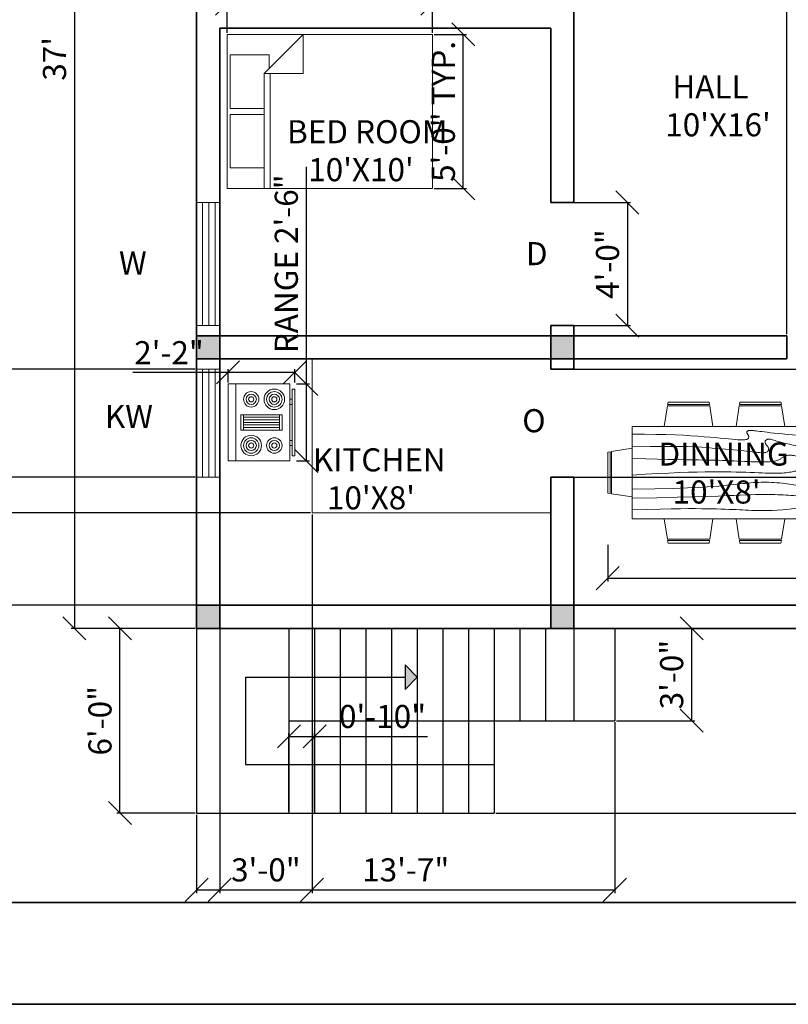
# Model space of a CAD drawing. Units: inches. Extents: x 1798 to 3594, y 1405 to 2404.
# Tile 2 of 6: x 2157 to 2457, y 1405 to 1789. Entities that reach past the tile are written whole.
import ezdxf

# ---------------------------------------------------------------- set-up
doc = ezdxf.new("R2010")
doc.units = ezdxf.units.IN
for name, color, linetype, lineweight in [('A-ANNO-DIMS', 6, 'Continuous', 18), ('A-ANNO-TEXT', 7, 'Continuous', 18), ('A-ANNO-TTLB', 7, 'Continuous', 35), ('A-AREA-IDEN', 242, 'Continuous', 18), ('A-EQPM', 51, 'Continuous', 18), ('A-FLOR-CASE', 51, 'Continuous', 18), ('A-FLOR-STRS', 7, 'Continuous', 25), ('A-FURN', 18, 'Continuous', 18), ('A-GLAZ', 4, 'Continuous', 18), ('A-WALL', 7, 'Continuous', 35), ('S-COLS', 1, 'Continuous', 35)]:
    doc.layers.add(name, color=color, linetype=linetype, lineweight=lineweight)
doc.styles.get("Standard").update_dxf_attribs({"font": 'arial.ttf'})
doc.dimstyles.new('ISO-25', dxfattribs={"dimtxt": 9, "dimasz": 9, "dimexe": 1.25, "dimexo": 0.625, "dimgap": 2, "dimtad": 1, "dimdec": 1, "dimlunit": 4, "dimtxsty": 'Standard', "dimblk": 'OBLIQUE', "dimcen": 2.5, "dimazin": 0, "dimtfac": 1, "dimtdec": 1, "dimtmove": 0, "dimatfit": 3, "dimfxl": 1, "dimarcsym": 0})

# ---------------------------------------------------------------- blocks, each defined once
blk = doc.blocks.new('_Oblique')
at = {"color": 0, "linetype": 'ByBlock', "lineweight": -2}
blk.add_line((-0.5, -0.5), (0.5, 0.5), dxfattribs=at)
blk = doc.blocks.new('*D3')
at = {"layer": 'A-ANNO-DIMS', "color": 0, "lineweight": -2, "transparency": 16777216}
for p, q in [((2225.65, 1995.81), (2177.4, 1995.81)), ((2178.65, 1995.81), (2178.65, 1551.81)), ((2225.65, 1551.81), (2177.4, 1551.81))]:
    blk.add_line(p, q, dxfattribs=at)
at = {"layer": 'Defpoints', "color": 0, "transparency": 16777216}
for p in [(2226.27, 1995.81), (2178.65, 1551.81), (2226.27, 1551.81)]:
    blk.add_point(p, dxfattribs=at)
at = {"layer": 'A-ANNO-DIMS', "color": 0, "lineweight": -2, "transparency": 16777216, "xscale": 9, "yscale": 9, "zscale": 9}
for p, rotation in [((2178.65, 1995.81), 90), ((2178.65, 1551.81), 270)]:
    blk.add_blockref('_Oblique', p, dxfattribs=dict(at, rotation=rotation))
at = {"layer": 'A-ANNO-DIMS', "color": 0, "transparency": 16777216, "insert": (2172.06, 1773.81), "char_height": 9, "attachment_point": 5, "rotation": 90}
blk.add_mtext("37'", dxfattribs=at)
blk = doc.blocks.new('Range-Oven - 30 in top')
for p, q in [((0, -3), (30, -3)), ((12, -6), (18, -6)), ((13, -20), (13, -6)), ((14, -6), (14, -20)), ((15, -20), (15, -6)), ((16, -6), (16, -20)), ((17, -20), (17, -6)), ((18, -20), (12, -20)), ((6, -24), (6, -25)), ((8, -25), (8, -24)), ((22, -25), (22, -24)), ((24, -24), (24, -25))]:
    blk.add_line(p, q)
for points in [[(0, -24), (0, 0), (30, 0), (30, -24)], [(12, -21), (12, -5), (18, -5), (18, -21)], [(2, -26), (2, -25), (28, -25), (28, -26)]]:
    blk.add_lwpolyline(points, close=True)
for centre, radius in [((6, -9), 4), ((6, -9), 3), ((6, -9), 2), ((24, -9), 3), ((24, -9), 2), ((6, -9), 1), ((24, -9), 1), ((6, -18), 3), ((24, -18), 4), ((24, -18), 3), ((6, -18), 2), ((6, -18), 1), ((24, -18), 2), ((24, -18), 1)]:
    blk.add_circle(centre, radius)
blk = doc.blocks.new('Bed - Queen')
for p, q in [((0, -80.00003), (0, 0)), ((0, 0), (59.99999, 0)), ((59.99999, 0), (59.99999, -80.00003)), ((7.99999, -1.2), (28.79998, -1.2)), ((7.99999, -14.4), (7.99999, -1.2)), ((28.79998, -1.2), (28.79998, -14.4)), ((31.19999, -1.2), (51.99999, -1.2)), ((31.19999, -14.4), (31.19999, -1.2)), ((51.99999, -1.2), (51.99999, -16.4)), ((0, -14.4), (44.8, -14.4)), ((59.99999, -29.6), (44.8, -14.4)), ((44.8, -14.4), (44.8, -29.6)), ((44.8, -16.8), (0, -16.8)), ((51.99999, -16.4), (46.79936, -16.4)), ((44.8, -29.6), (59.99999, -29.6)), ((59.99999, -80.00003), (0, -80.00003))]:
    blk.add_line(p, q)
blk = doc.blocks.new('Dining Set - 36 x 72 in.')
for p, q in [((-22, 27.5), (-22.1562, 26.50042)), ((-22, 27.5), (-6, 27.5)), ((-5.8437, 26.49966), (-6, 27.5)), ((6, 27.5), (5.8438, 26.50042)), ((6, 27.5), (22, 27.5)), ((22.1563, 26.49966), (22, 27.5)), ((-22.2343, 26.00059), (-23.4847, 17.99762)), ((-22.2304, 26), (-5.7608, 26)), ((-5.8416, 26.5), (-22.1534, 26.5)), ((-4.5152, 17.99762), (-5.7655, 25.99926)), ((5.7657, 26.00059), (4.5153, 17.99762)), ((5.7696, 26), (22.2392, 26)), ((22.1584, 26.5), (5.8466, 26.5)), ((23.4848, 17.99762), (22.2345, 25.99926)), ((36, 18), (-36, 18)), ((-36, 18), (-36, -18)), ((36, -18), (36, 18)), ((-45.5, 8), (-44.5004, 8.15617)), ((-45.5, 8), (-45.5, -8)), ((-44.5, -8.15843), (-44.5, 8.15338)), ((-44.0006, 8.23428), (-35.9976, 9.48474)), ((-44, 8.23041), (-44, -8.23915)), ((44.0006, 8.23428), (35.9976, 9.48474)), ((44, 8.23041), (44, -8.23915)), ((44.5, -8.15843), (44.5, 8.15338)), ((45.5, 8), (44.5005, 8.15617)), ((45.5, 8), (45.5, -8)), ((-44.4997, -8.15631), (-45.5, -8)), ((-35.9976, -9.48476), (-43.9993, -8.2345)), ((35.9976, -9.48476), (43.9993, -8.2345)), ((44.4997, -8.15631), (45.5, -8)), ((-36, -18), (36, -18)), ((-22.2343, -26.0006), (-23.4847, -17.99762)), ((-4.5152, -17.99762), (-5.7655, -25.99928)), ((5.7657, -26.0006), (4.5153, -17.99762)), ((23.4848, -17.99762), (22.2345, -25.99928)), ((-22.2304, -26), (-5.7608, -26)), ((-22, -27.5), (-22.1562, -26.50044)), ((-5.8416, -26.5), (-22.1534, -26.5)), ((-5.8437, -26.49967), (-6, -27.5)), ((5.7696, -26), (22.2392, -26)), ((6, -27.5), (5.8438, -26.50044)), ((22.1584, -26.5), (5.8466, -26.5)), ((22.1563, -26.49967), (22, -27.5)), ((-22, -27.5), (-6, -27.5)), ((6, -27.5), (22, -27.5))]:
    blk.add_line(p, q)
for points in [[(-36, 15), (-31.1772, 14.97754), (-26.8079, 14.91406), (-22.8538, 14.81543), (-19.276, 14.6875), (-16.0362, 14.53613), (-13.0957, 14.36718), (-10.4159, 14.18652), (-7.9583, 14), (-5.6904, 13.81315), (-3.6035, 13.63021), (-1.6954, 13.45508), (0.0365, 13.29166), (1.5945, 13.14388), (2.9811, 13.01562), (4.1988, 12.9108), (5.25, 12.83333), (6.1393, 12.78613), (6.8802, 12.76823), (7.4883, 12.77767), (7.9792, 12.8125), (8.3685, 12.87077), (8.6719, 12.95052), (8.9049, 13.0498), (9.0833, 13.16666), (9.2205, 13.29899), (9.3216, 13.44401), (9.3895, 13.59879), (9.4271, 13.76041), (9.4373, 13.92594), (9.4232, 14.09245), (9.3875, 14.257), (9.3333, 14.41666), (9.2638, 14.56917), (9.1836, 14.71484), (9.0975, 14.85465), (9.0104, 14.98958), (8.9272, 15.1206), (8.8529, 15.2487), (8.7922, 15.37483), (8.75, 15.5), (8.7305, 15.62467), (8.7344, 15.74739), (8.7617, 15.86621), (8.8125, 15.97916), (8.8867, 16.08431), (8.9844, 16.17968), (9.1055, 16.26334), (9.25, 16.33333), (9.4189, 16.38802), (9.6172, 16.42708), (9.8506, 16.45052), (10.125, 16.45833), (10.4463, 16.45052), (10.8203, 16.42708), (11.2529, 16.38802), (11.75, 16.33333), (12.3184, 16.26318), (12.9694, 16.17838), (13.7151, 16.07991), (14.5677, 15.96875), (15.5395, 15.84586), (16.6426, 15.71224), (17.8893, 15.56884), (19.2917, 15.41666), (20.859, 15.25667), (22.5879, 15.08984), (24.4721, 14.91715), (26.5052, 14.73958), (28.6809, 14.5581), (30.9929, 14.3737), (33.4347, 14.18733), (36, 14)], [(-36, 10), (-28.9766, 10.14274), (-23.1725, 10.20442), (-18.4241, 10.19775), (-14.5677, 10.13541), (-11.4399, 10.03011), (-8.877, 9.89453), (-6.7154, 9.74137), (-4.7917, 9.58333), (-2.9698, 9.43082), (-1.2246, 9.28515), (0.4415, 9.14534), (2.026, 9.01041), (3.5266, 8.87939), (4.9408, 8.7513), (6.266, 8.62516), (7.5, 8.5), (8.6411, 8.37549), (9.6914, 8.2539), (10.6538, 8.13818), (11.5312, 8.03125), (12.3267, 7.93603), (13.043, 7.85547), (13.6831, 7.79248), (14.25, 7.75), (14.7471, 7.7303), (15.1797, 7.73307), (15.5537, 7.75732), (15.875, 7.80208), (16.1494, 7.86637), (16.3828, 7.94922), (16.5811, 8.04964), (16.75, 8.16666), (16.8944, 8.29915), (17.0143, 8.44531), (17.1089, 8.60319), (17.1771, 8.77083), (17.218, 8.94629), (17.2305, 9.1276), (17.2137, 9.31282), (17.1667, 9.5), (17.0895, 9.6875), (16.987, 9.875), (16.8649, 10.0625), (16.7292, 10.25), (16.5856, 10.4375), (16.4401, 10.625), (16.2985, 10.8125), (16.1667, 11), (16.05, 11.18733), (15.9518, 11.3737), (15.8752, 11.5581), (15.8229, 11.73958), (15.798, 11.91715), (15.8034, 12.08984), (15.842, 12.25667), (15.9167, 12.41666), (16.0295, 12.56836), (16.1784, 12.70833), (16.3605, 12.83268), (16.5729, 12.9375), (16.8127, 13.01888), (17.0768, 13.07291), (17.3625, 13.0957), (17.6667, 13.08333), (17.9894, 13.03312), (18.3418, 12.94726), (18.7382, 12.82918), (19.1927, 12.68229), (19.7195, 12.51001), (20.3327, 12.31575), (21.0465, 12.10294), (21.875, 11.875), (22.8357, 11.63354), (23.959, 11.37304), (25.2786, 11.08618), (26.8282, 10.76562), (28.6414, 10.40405), (30.752, 9.99414), (33.1936, 9.52856), (36, 9)], [(-36, 5.5), (-30.7157, 5.3348), (-26.069, 5.20963), (-21.9946, 5.11767), (-18.4271, 5.05208), (-15.3009, 5.00602), (-12.5508, 4.97265), (-10.1112, 4.94515), (-7.9167, 4.91666), (-5.909, 4.88167), (-4.0586, 4.83984), (-2.3429, 4.79215), (-0.7396, 4.73958), (0.7739, 4.6831), (2.22, 4.6237), (3.6213, 4.56233), (5, 4.5), (6.373, 4.43782), (7.7344, 4.3776), (9.0723, 4.32129), (10.375, 4.27083), (11.6309, 4.22819), (12.8281, 4.19531), (13.9551, 4.17415), (15, 4.16666), (15.954, 4.17448), (16.819, 4.19791), (17.6001, 4.23698), (18.3021, 4.29166), (18.9299, 4.36198), (19.4883, 4.44791), (19.9823, 4.54948), (20.4167, 4.66666), (20.7969, 4.79899), (21.1302, 4.94401), (21.4245, 5.09879), (21.6875, 5.26041), (21.9271, 5.42594), (22.1511, 5.59245), (22.3672, 5.757), (22.5834, 5.91666), (22.8065, 6.06868), (23.0404, 6.21093), (23.2879, 6.34147), (23.5521, 6.45833), (23.8358, 6.55957), (24.142, 6.64323), (24.4735, 6.70735), (24.8334, 6.75), (25.2235, 6.76969), (25.642, 6.76692), (26.0858, 6.74267), (26.5521, 6.69791), (27.0379, 6.63362), (27.5404, 6.55078), (28.0565, 6.45036), (28.5834, 6.33333), (29.1242, 6.19987), (29.7071, 6.04687), (30.3661, 5.87044), (31.1354, 5.66666), (32.0493, 5.43164), (33.142, 5.16146), (34.4475, 4.85221), (36, 4.5)], [(-36, -1), (-30.7915, -0.6591), (-26.0195, -0.38216), (-21.6519, -0.16284), (-17.6563, 0.00521), (-14.0005, 0.12833), (-10.6523, 0.21289), (-7.5796, 0.26522), (-4.75, 0.29166), (-2.134, 0.29793), (0.2878, 0.28711), (2.5317, 0.26163), (4.6146, 0.22396), (6.5529, 0.17651), (8.3633, 0.12174), (10.0623, 0.06209), (11.6667, 0), (13.1899, -0.06201), (14.6341, -0.1211), (15.9982, -0.17432), (17.2813, -0.21875), (18.4823, -0.25147), (19.6003, -0.26953), (20.6343, -0.27002), (21.5834, -0.25), (22.4481, -0.20768), (23.2357, -0.14584), (23.9549, -0.06836), (24.6146, 0.02083), (25.2235, 0.11784), (25.7904, 0.21875), (26.3241, 0.31966), (26.8334, 0.41666), (27.3265, 0.50618), (27.8099, 0.58593), (28.2894, 0.65397), (28.7709, 0.70833), (29.2601, 0.74707), (29.763, 0.76823), (30.2855, 0.76985), (30.8334, 0.75), (31.4088, 0.70784), (31.9994, 0.64713), (32.589, 0.57275), (33.1615, 0.48958), (33.7008, 0.4025), (34.1908, 0.3164), (34.6153, 0.23616), (34.9584, 0.16666), (35.2099, 0.11165), (35.3848, 0.07031), (35.504, 0.04069), (35.5886, 0.02083), (35.6594, 0.00879), (35.7377, 0.0026), (35.8442, 0.00032), (36, 0)], [(-36, -6.5), (-27.1843, -6.31267), (-20.084, -6.1263), (-14.469, -5.9419), (-10.1094, -5.76042), (-6.7752, -5.58285), (-4.2363, -5.41016), (-2.2629, -5.24333), (-0.625, -5.08334), (0.8708, -4.93099), (2.2715, -4.78646), (3.5872, -4.64974), (4.8281, -4.52084), (6.0046, -4.39974), (7.127, -4.28646), (8.2053, -4.18099), (9.25, -4.08334), (10.2705, -3.99382), (11.2734, -3.91407), (12.2647, -3.84603), (13.25, -3.79167), (14.2354, -3.75293), (15.2266, -3.73177), (16.2295, -3.73015), (17.25, -3.75), (18.2912, -3.79248), (19.3451, -3.85547), (20.4009, -3.93604), (21.4479, -4.03125), (22.4754, -4.13819), (23.4727, -4.25391), (24.4289, -4.37549), (25.3334, -4.5), (26.1785, -4.62492), (26.9694, -4.74935), (27.7145, -4.87281), (28.4219, -4.99479), (29.1, -5.11483), (29.7572, -5.23242), (30.4016, -5.34709), (31.0417, -5.45834), (31.6837, -5.56437), (32.3262, -5.65821), (32.9658, -5.73153), (33.599, -5.77604), (34.2224, -5.78345), (34.8327, -5.74545), (35.4264, -5.65373), (36, -5.5)], [(-36, -10), (-26.4022, -9.81299), (-18.4675, -9.62891), (-11.9839, -9.45069), (-6.7396, -9.28125), (-2.5226, -9.12354), (0.8789, -8.98047), (3.6769, -8.85498), (6.0833, -8.75), (8.2767, -8.66765), (10.3021, -8.60677), (12.1712, -8.56543), (13.8958, -8.54167), (15.4876, -8.53353), (16.9583, -8.53907), (18.3197, -8.55632), (19.5834, -8.58334), (20.7616, -8.61841), (21.8685, -8.66081), (22.9188, -8.71004), (23.9271, -8.76563), (24.9081, -8.82707), (25.8763, -8.89388), (26.8465, -8.96558), (27.8334, -9.04167), (28.8474, -9.12118), (29.8828, -9.20117), (30.93, -9.27824), (31.9792, -9.34896), (33.0205, -9.40991), (34.0443, -9.45768), (35.0407, -9.48885), (36, -9.5)], [(-36, -14.5), (-30.0881, -14.33513), (-25.0332, -14.21224), (-20.7312, -14.12647), (-17.0781, -14.07292), (-13.97, -14.04671), (-11.3027, -14.04297), (-8.9724, -14.05681), (-6.875, -14.08334), (-4.9224, -14.11833), (-3.0905, -14.16016), (-1.3709, -14.20785), (0.2448, -14.26042), (1.7647, -14.3169), (3.1973, -14.3763), (4.5507, -14.43767), (5.8333, -14.5), (7.0554, -14.5621), (8.235, -14.62175), (9.3922, -14.67652), (10.5469, -14.72396), (11.7192, -14.76164), (12.929, -14.78711), (14.1965, -14.79794), (15.5417, -14.79167), (16.9933, -14.76424), (18.6152, -14.70508), (20.4804, -14.60197), (22.6615, -14.44271), (25.2312, -14.21509), (28.2624, -13.9069), (31.8277, -13.50594), (36, -13)]]:
    blk.add_lwpolyline(points)
blk = doc.blocks.new('COLUMN-9X9')
h = blk.add_hatch(color=256)
h.dxf.hatch_style = 1
h.paths.add_polyline_path([(9, 9), (0, 9), (0, 0), (9, 0)])
blk.add_lwpolyline([(0, 9), (9, 9), (9, 0), (0, 0)], close=True)
blk = doc.blocks.new('WINDOW-48-PLAN')
for p, q in [((0, 48), (9, 48)), ((2.25, 48), (2.25, 0)), ((4.75, 48), (4.75, 0)), ((7.25, 48), (7.25, 0)), ((7.25, 48), (7.25, 0)), ((0, 0), (9, 0))]:
    blk.add_line(p, q)
blk = doc.blocks.new('*D19')
at = {"layer": 'A-ANNO-DIMS', "color": 0, "lineweight": -2, "transparency": 16777216}
for p, q in [((2238.18, 1783.93), (2238.18, 1796.56)), ((2318.18, 1783.93), (2318.18, 1796.56)), ((2238.18, 1795.31), (2092.79, 1795.31)), ((2318.18, 1795.31), (2238.18, 1795.31))]:
    blk.add_line(p, q, dxfattribs=at)
at = {"layer": 'Defpoints', "color": 0, "transparency": 16777216}
for p in [(2238.18, 1795.31), (2238.18, 1783.31), (2318.18, 1783.31)]:
    blk.add_point(p, dxfattribs=at)
at = {"layer": 'A-ANNO-DIMS', "color": 0, "lineweight": -2, "transparency": 16777216, "xscale": 9, "yscale": 9, "zscale": 9, "rotation": 180}
blk.add_blockref('_Oblique', (2238.18, 1795.31), dxfattribs=at)
at = {"layer": 'A-ANNO-DIMS', "color": 0, "lineweight": -2, "transparency": 16777216, "xscale": 9, "yscale": 9, "zscale": 9}
blk.add_blockref('_Oblique', (2318.18, 1795.31), dxfattribs=at)
at = {"layer": 'A-ANNO-DIMS', "color": 0, "transparency": 16777216, "insert": (2160.99, 1802.24), "char_height": 9, "attachment_point": 5}
blk.add_mtext('QUEEN BED 6\'-8" TYP.', dxfattribs=at)
blk = doc.blocks.new('*D20')
at = {"layer": 'A-ANNO-DIMS', "color": 0, "lineweight": -2, "transparency": 16777216}
for p, q in [((2318.81, 1783.31), (2331.43, 1783.31)), ((2330.18, 1723.31), (2330.18, 1783.31)), ((2318.81, 1723.31), (2331.43, 1723.31))]:
    blk.add_line(p, q, dxfattribs=at)
at = {"layer": 'Defpoints', "color": 0, "transparency": 16777216}
for p in [(2318.18, 1783.31), (2330.18, 1783.31), (2318.18, 1723.31)]:
    blk.add_point(p, dxfattribs=at)
at = {"layer": 'A-ANNO-DIMS', "color": 0, "lineweight": -2, "transparency": 16777216, "xscale": 9, "yscale": 9, "zscale": 9}
for p, rotation in [((2330.18, 1783.31), 90), ((2330.18, 1723.31), 270)]:
    blk.add_blockref('_Oblique', p, dxfattribs=dict(at, rotation=rotation))
at = {"layer": 'A-ANNO-DIMS', "color": 0, "transparency": 16777216, "insert": (2323.59, 1753.31), "char_height": 9, "attachment_point": 5, "rotation": 90}
blk.add_mtext('5\'-0" TYP.', dxfattribs=at)
blk = doc.blocks.new('*D25')
at = {"layer": 'A-ANNO-DIMS', "color": 0, "lineweight": -2, "transparency": 16777216}
for p, q in [((2269.05, 1647.09), (2269.05, 1731.75)), ((2265.17, 1647.09), (2270.3, 1647.09)), ((2269.05, 1617.09), (2269.05, 1647.09)), ((2265.17, 1617.09), (2270.3, 1617.09))]:
    blk.add_line(p, q, dxfattribs=at)
at = {"layer": 'Defpoints', "color": 0, "transparency": 16777216}
for p in [(2264.55, 1647.09), (2269.05, 1647.09), (2264.55, 1617.09)]:
    blk.add_point(p, dxfattribs=at)
at = {"layer": 'A-ANNO-DIMS', "color": 0, "lineweight": -2, "transparency": 16777216, "xscale": 9, "yscale": 9, "zscale": 9}
for p, rotation in [((2269.05, 1647.09), 90), ((2269.05, 1617.09), 270)]:
    blk.add_blockref('_Oblique', p, dxfattribs=dict(at, rotation=rotation))
at = {"layer": 'A-ANNO-DIMS', "color": 0, "transparency": 16777216, "insert": (2262.39, 1693.92), "char_height": 9, "attachment_point": 5, "rotation": 90}
blk.add_mtext('RANGE 2\'-6"', dxfattribs=at)
blk = doc.blocks.new('*D26')
at = {"layer": 'A-ANNO-DIMS', "color": 0, "lineweight": -2, "transparency": 16777216}
for p, q in [((2238.55, 1651.59), (2201.47, 1651.59)), ((2238.55, 1647.71), (2238.55, 1652.84)), ((2264.55, 1651.59), (2238.55, 1651.59)), ((2264.55, 1647.71), (2264.55, 1652.84))]:
    blk.add_line(p, q, dxfattribs=at)
at = {"layer": 'Defpoints', "color": 0, "transparency": 16777216}
for p in [(2238.55, 1651.59), (2238.55, 1647.09), (2264.55, 1647.09)]:
    blk.add_point(p, dxfattribs=at)
at = {"layer": 'A-ANNO-DIMS', "color": 0, "lineweight": -2, "transparency": 16777216, "xscale": 9, "yscale": 9, "zscale": 9, "rotation": 180}
blk.add_blockref('_Oblique', (2238.55, 1651.59), dxfattribs=at)
at = {"layer": 'A-ANNO-DIMS', "color": 0, "lineweight": -2, "transparency": 16777216, "xscale": 9, "yscale": 9, "zscale": 9}
blk.add_blockref('_Oblique', (2264.55, 1651.59), dxfattribs=at)
at = {"layer": 'A-ANNO-DIMS', "color": 0, "transparency": 16777216, "insert": (2215.51, 1658.1), "char_height": 9, "attachment_point": 5}
blk.add_mtext('2\'-2"', dxfattribs=at)
blk = doc.blocks.new('*D27')
at = {"layer": 'A-ANNO-DIMS', "color": 0, "lineweight": -2, "transparency": 16777216}
for p, q in [((2386.49, 1584.39), (2386.49, 1570.12)), ((2477.49, 1584.39), (2477.49, 1570.12)), ((2386.49, 1571.37), (2477.49, 1571.37)), ((2477.49, 1571.37), (2589.41, 1571.37))]:
    blk.add_line(p, q, dxfattribs=at)
at = {"layer": 'Defpoints', "color": 0, "transparency": 16777216}
for p in [(2386.49, 1585.02), (2477.49, 1585.02), (2477.49, 1571.37)]:
    blk.add_point(p, dxfattribs=at)
at = {"layer": 'A-ANNO-DIMS', "color": 0, "lineweight": -2, "transparency": 16777216, "xscale": 9, "yscale": 9, "zscale": 9, "rotation": 180}
blk.add_blockref('_Oblique', (2386.49, 1571.37), dxfattribs=at)
at = {"layer": 'A-ANNO-DIMS', "color": 0, "lineweight": -2, "transparency": 16777216, "xscale": 9, "yscale": 9, "zscale": 9}
blk.add_blockref('_Oblique', (2477.49, 1571.37), dxfattribs=at)
at = {"layer": 'A-ANNO-DIMS', "color": 0, "transparency": 16777216, "insert": (2537.95, 1578.02), "char_height": 9, "attachment_point": 5}
blk.add_mtext('DINING SET 7\'-7"', dxfattribs=at)
blk = doc.blocks.new('*D29')
at = {"layer": 'A-ANNO-DIMS', "color": 0, "lineweight": -2, "transparency": 16777216}
for p, q in [((2225.65, 1551.81), (2195.12, 1551.81)), ((2196.37, 1479.81), (2196.37, 1551.81)), ((2225.65, 1479.81), (2195.12, 1479.81))]:
    blk.add_line(p, q, dxfattribs=at)
at = {"layer": 'Defpoints', "color": 0, "transparency": 16777216}
for p in [(2196.37, 1551.81), (2226.27, 1551.81), (2226.27, 1479.81)]:
    blk.add_point(p, dxfattribs=at)
at = {"layer": 'A-ANNO-DIMS', "color": 0, "lineweight": -2, "transparency": 16777216, "xscale": 9, "yscale": 9, "zscale": 9}
for p, rotation in [((2196.37, 1551.81), 90), ((2196.37, 1479.81), 270)]:
    blk.add_blockref('_Oblique', p, dxfattribs=dict(at, rotation=rotation))
at = {"layer": 'A-ANNO-DIMS', "color": 0, "transparency": 16777216, "insert": (2189.78, 1515.81), "char_height": 9, "attachment_point": 5, "rotation": 90}
blk.add_mtext('6\'-0"', dxfattribs=at)
blk = doc.blocks.new('*D30')
at = {"layer": 'A-ANNO-DIMS', "color": 0, "lineweight": -2, "transparency": 16777216}
for p, q in [((2511.9, 1995.81), (2542.42, 1995.81)), ((2541.17, 1479.81), (2541.17, 1995.81)), ((2342.9, 1479.81), (2542.42, 1479.81))]:
    blk.add_line(p, q, dxfattribs=at)
at = {"layer": 'Defpoints', "color": 0, "transparency": 16777216}
for p in [(2511.27, 1995.81), (2541.17, 1995.81), (2342.27, 1479.81)]:
    blk.add_point(p, dxfattribs=at)
at = {"layer": 'A-ANNO-DIMS', "color": 0, "lineweight": -2, "transparency": 16777216, "xscale": 9, "yscale": 9, "zscale": 9}
for p, rotation in [((2541.17, 1995.81), 90), ((2541.17, 1479.81), 270)]:
    blk.add_blockref('_Oblique', p, dxfattribs=dict(at, rotation=rotation))
at = {"layer": 'A-ANNO-DIMS', "color": 0, "transparency": 16777216, "insert": (2534.57, 1737.81), "char_height": 9, "attachment_point": 5, "rotation": 90}
blk.add_mtext('43\'-0"', dxfattribs=at)
blk = doc.blocks.new('*D31')
at = {"layer": 'A-ANNO-DIMS', "color": 0, "lineweight": -2, "transparency": 16777216}
for p, q in [((2389.27, 1515.19), (2389.27, 1448.66)), ((2226.27, 1479.19), (2226.27, 1448.66)), ((2226.27, 1449.91), (2389.27, 1449.91))]:
    blk.add_line(p, q, dxfattribs=at)
at = {"layer": 'Defpoints', "color": 0, "transparency": 16777216}
for p in [(2389.27, 1515.81), (2226.27, 1479.81), (2389.27, 1449.91)]:
    blk.add_point(p, dxfattribs=at)
at = {"layer": 'A-ANNO-DIMS', "color": 0, "lineweight": -2, "transparency": 16777216, "xscale": 9, "yscale": 9, "zscale": 9, "rotation": 180}
blk.add_blockref('_Oblique', (2226.27, 1449.91), dxfattribs=at)
at = {"layer": 'A-ANNO-DIMS', "color": 0, "lineweight": -2, "transparency": 16777216, "xscale": 9, "yscale": 9, "zscale": 9}
blk.add_blockref('_Oblique', (2389.27, 1449.91), dxfattribs=at)
at = {"layer": 'A-ANNO-DIMS', "color": 0, "transparency": 16777216, "insert": (2307.77, 1456.51), "char_height": 9, "attachment_point": 5}
blk.add_mtext('13\'-7"', dxfattribs=at)
blk = doc.blocks.new('*D32')
at = {"layer": 'A-ANNO-DIMS', "color": 0, "lineweight": -2, "transparency": 16777216}
for p, q in [((2389.9, 1551.81), (2420.42, 1551.81)), ((2419.17, 1551.81), (2419.17, 1515.81)), ((2389.9, 1515.81), (2420.42, 1515.81))]:
    blk.add_line(p, q, dxfattribs=at)
at = {"layer": 'Defpoints', "color": 0, "transparency": 16777216}
for p in [(2389.27, 1551.81), (2389.27, 1515.81), (2419.17, 1515.81)]:
    blk.add_point(p, dxfattribs=at)
at = {"layer": 'A-ANNO-DIMS', "color": 0, "lineweight": -2, "transparency": 16777216, "xscale": 9, "yscale": 9, "zscale": 9}
for p, rotation in [((2419.17, 1551.81), 90), ((2419.17, 1515.81), 270)]:
    blk.add_blockref('_Oblique', p, dxfattribs=dict(at, rotation=rotation))
at = {"layer": 'A-ANNO-DIMS', "color": 0, "transparency": 16777216, "insert": (2412.57, 1533.81), "char_height": 9, "attachment_point": 5, "rotation": 90}
blk.add_mtext('3\'-0"', dxfattribs=at)
blk = doc.blocks.new('*D33')
at = {"layer": 'A-ANNO-DIMS', "color": 0, "lineweight": -2, "transparency": 16777216}
for p, q in [((2262.27, 1480.44), (2262.27, 1510.96)), ((2262.27, 1509.71), (2272.27, 1509.71)), ((2272.27, 1480.44), (2272.27, 1510.96)), ((2272.27, 1509.71), (2316.19, 1509.71))]:
    blk.add_line(p, q, dxfattribs=at)
at = {"layer": 'Defpoints', "color": 0, "transparency": 16777216}
for p in [(2272.27, 1509.71), (2262.27, 1479.81), (2272.27, 1479.81)]:
    blk.add_point(p, dxfattribs=at)
at = {"layer": 'A-ANNO-DIMS', "color": 0, "lineweight": -2, "transparency": 16777216, "xscale": 9, "yscale": 9, "zscale": 9, "rotation": 180}
blk.add_blockref('_Oblique', (2262.27, 1509.71), dxfattribs=at)
at = {"layer": 'A-ANNO-DIMS', "color": 0, "lineweight": -2, "transparency": 16777216, "xscale": 9, "yscale": 9, "zscale": 9}
blk.add_blockref('_Oblique', (2272.27, 1509.71), dxfattribs=at)
at = {"layer": 'A-ANNO-DIMS', "color": 0, "transparency": 16777216, "insert": (2298.73, 1516.31), "char_height": 9, "attachment_point": 5}
blk.add_mtext('0\'-10"', dxfattribs=at)
blk = doc.blocks.new('*D41')
at = {"layer": 'A-ANNO-DIMS', "color": 0, "lineweight": -2, "transparency": 16777216}
for p, q in [((2364.9, 1717.81), (2395.42, 1717.81)), ((2394.17, 1717.81), (2394.17, 1669.81)), ((2364.9, 1669.81), (2395.42, 1669.81))]:
    blk.add_line(p, q, dxfattribs=at)
at = {"layer": 'Defpoints', "color": 0, "transparency": 16777216}
for p in [(2364.27, 1717.81), (2364.27, 1669.81), (2394.17, 1669.81)]:
    blk.add_point(p, dxfattribs=at)
at = {"layer": 'A-ANNO-DIMS', "color": 0, "lineweight": -2, "transparency": 16777216, "xscale": 9, "yscale": 9, "zscale": 9}
for p, rotation in [((2394.17, 1717.81), 90), ((2394.17, 1669.81), 270)]:
    blk.add_blockref('_Oblique', p, dxfattribs=dict(at, rotation=rotation))
at = {"layer": 'A-ANNO-DIMS', "color": 0, "transparency": 16777216, "insert": (2387.58, 1693.81), "char_height": 9, "attachment_point": 5, "rotation": 90}
blk.add_mtext('4\'-0"', dxfattribs=at)
blk = doc.blocks.new('*D46')
at = {"layer": 'A-ANNO-DIMS', "color": 0, "lineweight": -2, "transparency": 16777216}
for p, q in [((2364.9, 1652.81), (2542.42, 1652.81)), ((2541.17, 1610.81), (2541.17, 1652.81)), ((2364.9, 1610.81), (2542.42, 1610.81))]:
    blk.add_line(p, q, dxfattribs=at)
at = {"layer": 'Defpoints', "color": 0, "transparency": 16777216}
for p in [(2364.27, 1652.81), (2541.17, 1652.81), (2364.27, 1610.81)]:
    blk.add_point(p, dxfattribs=at)
at = {"layer": 'A-ANNO-DIMS', "color": 0, "lineweight": -2, "transparency": 16777216, "xscale": 9, "yscale": 9, "zscale": 9}
for p, rotation in [((2541.17, 1652.81), 90), ((2541.17, 1610.81), 270)]:
    blk.add_blockref('_Oblique', p, dxfattribs=dict(at, rotation=rotation))
at = {"layer": 'A-ANNO-DIMS', "color": 0, "transparency": 16777216, "insert": (2534.57, 1631.81), "char_height": 9, "attachment_point": 5, "rotation": 90}
blk.add_mtext('3\'-6"', dxfattribs=at)
blk = doc.blocks.new('*D47')
at = {"layer": 'A-ANNO-DIMS', "color": 0, "lineweight": -2, "transparency": 16777216}
for p, q in [((2456.27, 1666.44), (2456.27, 2092.43)), ((2498.27, 1666.44), (2498.27, 2092.43)), ((2456.27, 2091.18), (2498.27, 2091.18))]:
    blk.add_line(p, q, dxfattribs=at)
at = {"layer": 'Defpoints', "color": 0, "transparency": 16777216}
for p in [(2498.27, 2091.18), (2456.27, 1665.81), (2498.27, 1665.81)]:
    blk.add_point(p, dxfattribs=at)
at = {"layer": 'A-ANNO-DIMS', "color": 0, "lineweight": -2, "transparency": 16777216, "xscale": 9, "yscale": 9, "zscale": 9, "rotation": 180}
blk.add_blockref('_Oblique', (2456.27, 2091.18), dxfattribs=at)
at = {"layer": 'A-ANNO-DIMS', "color": 0, "lineweight": -2, "transparency": 16777216, "xscale": 9, "yscale": 9, "zscale": 9}
blk.add_blockref('_Oblique', (2498.27, 2091.18), dxfattribs=at)
at = {"layer": 'A-ANNO-DIMS', "color": 0, "transparency": 16777216, "insert": (2477.27, 2097.78), "char_height": 9, "attachment_point": 5}
blk.add_mtext('3\'-6"', dxfattribs=at)
blk = doc.blocks.new('*D48')
at = {"layer": 'A-ANNO-DIMS', "color": 0, "lineweight": -2, "transparency": 16777216}
for p, q in [((2225.65, 1652.81), (2036.12, 1652.81)), ((2037.37, 1610.81), (2037.37, 1652.81)), ((2225.65, 1610.81), (2036.12, 1610.81))]:
    blk.add_line(p, q, dxfattribs=at)
at = {"layer": 'Defpoints', "color": 0, "transparency": 16777216}
for p in [(2037.37, 1652.81), (2226.27, 1652.81), (2226.27, 1610.81)]:
    blk.add_point(p, dxfattribs=at)
at = {"layer": 'A-ANNO-DIMS', "color": 0, "lineweight": -2, "transparency": 16777216, "xscale": 9, "yscale": 9, "zscale": 9}
for p, rotation in [((2037.37, 1652.81), 90), ((2037.37, 1610.81), 270)]:
    blk.add_blockref('_Oblique', p, dxfattribs=dict(at, rotation=rotation))
at = {"layer": 'A-ANNO-DIMS', "color": 0, "transparency": 16777216, "insert": (2030.77, 1631.81), "char_height": 9, "attachment_point": 5, "rotation": 90}
blk.add_mtext('3\'-6"', dxfattribs=at)
blk = doc.blocks.new('*D51')
at = {"layer": 'A-ANNO-DIMS', "color": 0, "lineweight": -2, "transparency": 16777216}
for p, q in [((2271.27, 1596.19), (2271.27, 1448.66)), ((2235.27, 1560.19), (2235.27, 1448.66)), ((2235.27, 1449.91), (2271.27, 1449.91))]:
    blk.add_line(p, q, dxfattribs=at)
at = {"layer": 'Defpoints', "color": 0, "transparency": 16777216}
for p in [(2271.27, 1596.81), (2235.27, 1560.81), (2271.27, 1449.91)]:
    blk.add_point(p, dxfattribs=at)
at = {"layer": 'A-ANNO-DIMS', "color": 0, "lineweight": -2, "transparency": 16777216, "xscale": 9, "yscale": 9, "zscale": 9, "rotation": 180}
blk.add_blockref('_Oblique', (2235.27, 1449.91), dxfattribs=at)
at = {"layer": 'A-ANNO-DIMS', "color": 0, "lineweight": -2, "transparency": 16777216, "xscale": 9, "yscale": 9, "zscale": 9}
blk.add_blockref('_Oblique', (2271.27, 1449.91), dxfattribs=at)
at = {"layer": 'A-ANNO-DIMS', "color": 0, "transparency": 16777216, "insert": (2253.27, 1456.51), "char_height": 9, "attachment_point": 5}
blk.add_mtext('3\'-0"', dxfattribs=at)
blk = doc.blocks.new('*D52')
at = {"layer": 'A-ANNO-DIMS', "color": 0, "lineweight": -2, "transparency": 16777216}
for p, q in [((2270.65, 1596.81), (2036.12, 1596.81)), ((2037.37, 1560.81), (2037.37, 1596.81)), ((2234.65, 1560.81), (2036.12, 1560.81))]:
    blk.add_line(p, q, dxfattribs=at)
at = {"layer": 'Defpoints', "color": 0, "transparency": 16777216}
for p in [(2037.37, 1596.81), (2271.27, 1596.81), (2235.27, 1560.81)]:
    blk.add_point(p, dxfattribs=at)
at = {"layer": 'A-ANNO-DIMS', "color": 0, "lineweight": -2, "transparency": 16777216, "xscale": 9, "yscale": 9, "zscale": 9}
for p, rotation in [((2037.37, 1596.81), 90), ((2037.37, 1560.81), 270)]:
    blk.add_blockref('_Oblique', p, dxfattribs=dict(at, rotation=rotation))
at = {"layer": 'A-ANNO-DIMS', "color": 0, "transparency": 16777216, "insert": (2030.77, 1578.81), "char_height": 9, "attachment_point": 5, "rotation": 90}
blk.add_mtext('3\'-0"', dxfattribs=at)

msp = doc.modelspace()

# ---------------------------------------------------------------- hatches: boundary and pattern name
at = {"layer": 'A-FLOR-STRS'}
h = msp.add_hatch(color=256, dxfattribs=at)
h.dxf.hatch_style = 1
h.paths.add_polyline_path([(2312.27, 1532.81), (2307.52, 1537.57), (2307.52, 1528.05)])

# ---------------------------------------------------------------- linework, layer by layer
at = {"layer": 'A-ANNO-TTLB'}
for points in [[(1798.35, 2403.73), (3594.23, 2403.73), (3594.23, 1405.28), (1798.35, 1405.28)], [(1855.68, 2366.05), (3540.6, 2366.05), (3540.6, 1444.98), (1855.68, 1444.98)]]:
    msp.add_lwpolyline(points, close=True, dxfattribs=at)
at = {"layer": 'A-FLOR-CASE'}
for p, q in [((2271.27, 1656.81), (2271.27, 1596.81)), ((2271.27, 1596.81), (2364.27, 1596.81))]:
    msp.add_line(p, q, dxfattribs=at)
at = {"layer": 'A-FLOR-STRS'}
for p, q in [((2226.27, 1551.81), (2226.27, 1479.81)), ((2226.27, 1551.81), (2226.27, 1479.81)), ((2235.27, 1551.81), (2235.27, 1479.81)), ((2262.27, 1551.81), (2262.27, 1479.81)), ((2272.27, 1551.81), (2272.27, 1479.81)), ((2282.27, 1551.81), (2282.27, 1479.81)), ((2292.27, 1551.81), (2292.27, 1479.81)), ((2302.27, 1551.81), (2302.27, 1479.81)), ((2312.27, 1551.81), (2312.27, 1479.81)), ((2322.27, 1551.81), (2322.27, 1479.81)), ((2332.27, 1551.81), (2332.27, 1479.81)), ((2342.27, 1551.81), (2342.27, 1479.81)), ((2352.27, 1551.81), (2352.27, 1515.81)), ((2362.27, 1551.81), (2362.27, 1515.81)), ((2373.27, 1551.81), (2373.27, 1515.81)), ((2389.27, 1551.81), (2389.27, 1515.81)), ((2312.27, 1532.81), (2307.52, 1537.57)), ((2312.27, 1532.81), (2307.52, 1537.57)), ((2312.27, 1532.81), (2307.52, 1537.57)), ((2307.52, 1537.57), (2307.52, 1528.05)), ((2245.27, 1532.81), (2307.52, 1532.81)), ((2245.27, 1532.81), (2245.27, 1498.81)), ((2312.27, 1532.81), (2307.52, 1528.05)), ((2262.27, 1515.81), (2389.27, 1515.81)), ((2245.27, 1498.81), (2342.27, 1498.81)), ((2226.27, 1479.81), (2342.27, 1479.81))]:
    msp.add_line(p, q, dxfattribs=at)
at = {"layer": 'A-GLAZ'}
for p, q in [((2226.27, 1669.81), (2235.27, 1669.81)), ((2226.27, 1652.81), (2235.27, 1652.81)), ((2228.52, 1652.81), (2228.52, 1610.81)), ((2231.02, 1652.81), (2231.02, 1610.81)), ((2233.52, 1652.81), (2233.52, 1610.81)), ((2233.52, 1652.81), (2233.52, 1610.81)), ((2226.27, 1610.81), (2235.27, 1610.81))]:
    msp.add_line(p, q, dxfattribs=at)
at = {"layer": 'A-WALL'}
for p, q in [((2226.27, 1995.81), (2226.27, 1551.81)), ((2373.27, 1794.81), (2373.27, 1717.81)), ((2235.27, 1785.81), (2364.27, 1785.81)), ((2235.27, 1785.81), (2235.27, 1551.81)), ((2364.27, 1785.81), (2364.27, 1717.81)), ((2364.27, 1717.81), (2373.27, 1717.81)), ((2364.27, 1669.81), (2364.27, 1656.81)), ((2364.27, 1669.81), (2373.27, 1669.81)), ((2373.27, 1669.81), (2373.27, 1656.81)), ((2226.27, 1665.81), (2364.27, 1665.81)), ((2364.27, 1665.81), (2456.27, 1665.81)), ((2456.27, 1665.81), (2456.27, 1656.81)), ((2226.27, 1656.81), (2364.27, 1656.81)), ((2364.27, 1656.81), (2364.27, 1652.81)), ((2373.27, 1656.81), (2373.27, 1652.81)), ((2373.27, 1656.81), (2456.27, 1656.81)), ((2364.27, 1652.81), (2373.27, 1652.81)), ((2364.27, 1610.81), (2364.27, 1560.81)), ((2364.27, 1610.81), (2373.27, 1610.81)), ((2373.27, 1610.81), (2373.27, 1560.81)), ((2226.27, 1560.81), (2511.27, 1560.81)), ((2226.27, 1551.81), (2511.27, 1551.81))]:
    msp.add_line(p, q, dxfattribs=at)

# ---------------------------------------------------------------- block references
at = {"layer": 'A-EQPM', "rotation": 90}
msp.add_blockref('Range-Oven - 30 in top', (2238.55, 1617.09), dxfattribs=at)
at = {"layer": 'A-FURN', "rotation": 90}
msp.add_blockref('Bed - Queen', (2238.18, 1723.31), dxfattribs=at)
at = {"layer": 'A-FURN'}
msp.add_blockref('Dining Set - 36 x 72 in.', (2431.99, 1612.52), dxfattribs=at)
at = {"layer": 'A-GLAZ'}
msp.add_blockref('WINDOW-48-PLAN', (2226.27, 1669.81), dxfattribs=at)
at = {"layer": 'S-COLS'}
for p in [(2226.27, 1656.81), (2364.27, 1656.81), (2226.27, 1551.81), (2364.27, 1551.81)]:
    msp.add_blockref('COLUMN-9X9', p, dxfattribs=at)

# ---------------------------------------------------------------- texts
at = {"layer": 'A-ANNO-TEXT'}
for s, p in [('               D', (2313.33, 1693.38)), ('               W', (2154.77, 1689.71)), ('             KW', (2154.77, 1629.88)), ('               O', (2311.92, 1628.26))]:
    msp.add_text(s, height=9, dxfattribs=at).set_placement(p)
at = {"layer": 'A-AREA-IDEN'}
for s, p in [('    HALL', (2400.66, 1758.39)), ('BED ROOM', (2261.52, 1740.89)), ("   10'X16'", (2400.66, 1743.6)), ("   10'X10'", (2261.52, 1726.1)), (' DINNING', (2403.52, 1615.26)), (' KITCHEN', (2268.82, 1612.99)), ("   10'X8'", (2403.52, 1600.47)), ("   10'X8'", (2268.82, 1598.2))]:
    msp.add_text(s, height=9, dxfattribs=at).set_placement(p)

# ---------------------------------------------------------------- dimensions: what is measured, and where the dimension line sits
at = {"layer": 'A-ANNO-DIMS'}
for base, p1, p2, picture, middle in [((2498.27, 2091.18), (2456.27, 1665.81), (2498.27, 1665.81), '*D47', (2477.27, 2097.78)), ((2271.27, 1449.91), (2235.27, 1560.81), (2271.27, 1596.81), '*D51', (2253.27, 1456.51)), ((2272.27, 1509.71), (2262.27, 1479.81), (2272.27, 1479.81), '*D33', (2298.73, 1516.31)), ((2389.27, 1449.91), (2226.27, 1479.81), (2389.27, 1515.81), '*D31', (2307.77, 1456.51))]:
    dim = msp.add_linear_dim(base=base, p1=p1, p2=p2, dimstyle='ISO-25', override={"dimdec": 1, "dimlfac": 1, "dimrnd": 0, "dimzin": 1, "dimdsep": 46, "dimlunit": 4, "dimfrac": 2}, dxfattribs=at)
    dim.commit()
    dim.dimension.update_dxf_attribs({"geometry": picture, "text_midpoint": middle})
for base, p1, p2, angle, override, picture, middle in [((2178.65, 1551.81), (2226.27, 1995.81), (2226.27, 1551.81), 90, {"dimclrd": 0, "dimclre": 0, "dimclrt": 0}, '*D3', (2172.06, 1773.81)), ((2541.17, 1995.81), (2342.27, 1479.81), (2511.27, 1995.81), 90, {"dimdec": 1, "dimlfac": 1, "dimrnd": 0, "dimzin": 1, "dimdsep": 46, "dimlunit": 4, "dimfrac": 2}, '*D30', (2534.57, 1737.81)), ((2394.17, 1669.81), (2364.27, 1717.81), (2364.27, 1669.81), 270, {"dimdec": 1, "dimlfac": 1, "dimrnd": 0, "dimzin": 1, "dimdsep": 46, "dimlunit": 4, "dimfrac": 2}, '*D41', (2387.58, 1693.81)), ((2238.55, 1651.59), (2264.55, 1647.09), (2238.55, 1647.09), 180, {"dimdec": 1, "dimlfac": 1, "dimrnd": 0, "dimzin": 1, "dimdsep": 46, "dimlunit": 4, "dimfrac": 2}, '*D26', (2215.51, 1658.1)), ((2037.37, 1652.81), (2226.27, 1610.81), (2226.27, 1652.81), 90, {"dimdec": 1, "dimlfac": 1, "dimrnd": 0, "dimzin": 1, "dimdsep": 46, "dimlunit": 4, "dimfrac": 2}, '*D48', (2030.77, 1631.81)), ((2541.17, 1652.81), (2364.27, 1610.81), (2364.27, 1652.81), 90, {"dimdec": 1, "dimlfac": 1, "dimrnd": 0, "dimzin": 1, "dimdsep": 46, "dimlunit": 4, "dimfrac": 2}, '*D46', (2534.57, 1631.81)), ((2037.37, 1596.81), (2235.27, 1560.81), (2271.27, 1596.81), 90, {"dimdec": 1, "dimlfac": 1, "dimrnd": 0, "dimzin": 1, "dimdsep": 46, "dimlunit": 4, "dimfrac": 2}, '*D52', (2030.77, 1578.81)), ((2196.37, 1551.81), (2226.27, 1479.81), (2226.27, 1551.81), 90, {"dimdec": 1, "dimlfac": 1, "dimrnd": 0, "dimzin": 1, "dimdsep": 46, "dimlunit": 4, "dimfrac": 2}, '*D29', (2189.78, 1515.81)), ((2419.17, 1515.81), (2389.27, 1551.81), (2389.27, 1515.81), 270, {"dimdec": 1, "dimlfac": 1, "dimrnd": 0, "dimzin": 1, "dimdsep": 46, "dimlunit": 4, "dimfrac": 2}, '*D32', (2412.57, 1533.81))]:
    dim = msp.add_linear_dim(base=base, p1=p1, p2=p2, angle=angle, dimstyle='ISO-25', override=override, dxfattribs=at)
    dim.commit()
    dim.dimension.update_dxf_attribs({"geometry": picture, "text_midpoint": middle})
for base, p1, p2, angle, text, picture, middle in [((2238.18, 1795.31), (2318.18, 1783.31), (2238.18, 1783.31), 180, 'QUEEN BED <> TYP.', '*D19', (2160.99, 1802.24)), ((2330.18, 1783.31), (2318.18, 1723.31), (2318.18, 1783.31), 90, '<> TYP.', '*D20', (2323.59, 1753.31)), ((2269.05, 1647.09), (2264.55, 1617.09), (2264.55, 1647.09), 90, 'RANGE <>', '*D25', (2262.39, 1693.92))]:
    dim = msp.add_linear_dim(base=base, p1=p1, p2=p2, angle=angle, text=text, dimstyle='ISO-25', override={"dimdec": 1, "dimlfac": 1, "dimrnd": 0, "dimzin": 1, "dimdsep": 46, "dimlunit": 4, "dimfrac": 2}, dxfattribs=at)
    dim.commit()
    dim.dimension.update_dxf_attribs({"geometry": picture, "text_midpoint": middle})
dim = msp.add_linear_dim(base=(2477.49, 1571.37), p1=(2386.49, 1585.02), p2=(2477.49, 1585.02), text='DINING SET <>', dimstyle='ISO-25', override={"dimdec": 1, "dimlfac": 1, "dimrnd": 0, "dimzin": 1, "dimdsep": 46, "dimlunit": 4, "dimfrac": 2}, dxfattribs=at)
dim.commit()
dim.dimension.update_dxf_attribs({"geometry": '*D27', "text_midpoint": (2537.95, 1578.02)})

doc.saveas('drawing.dxf')
